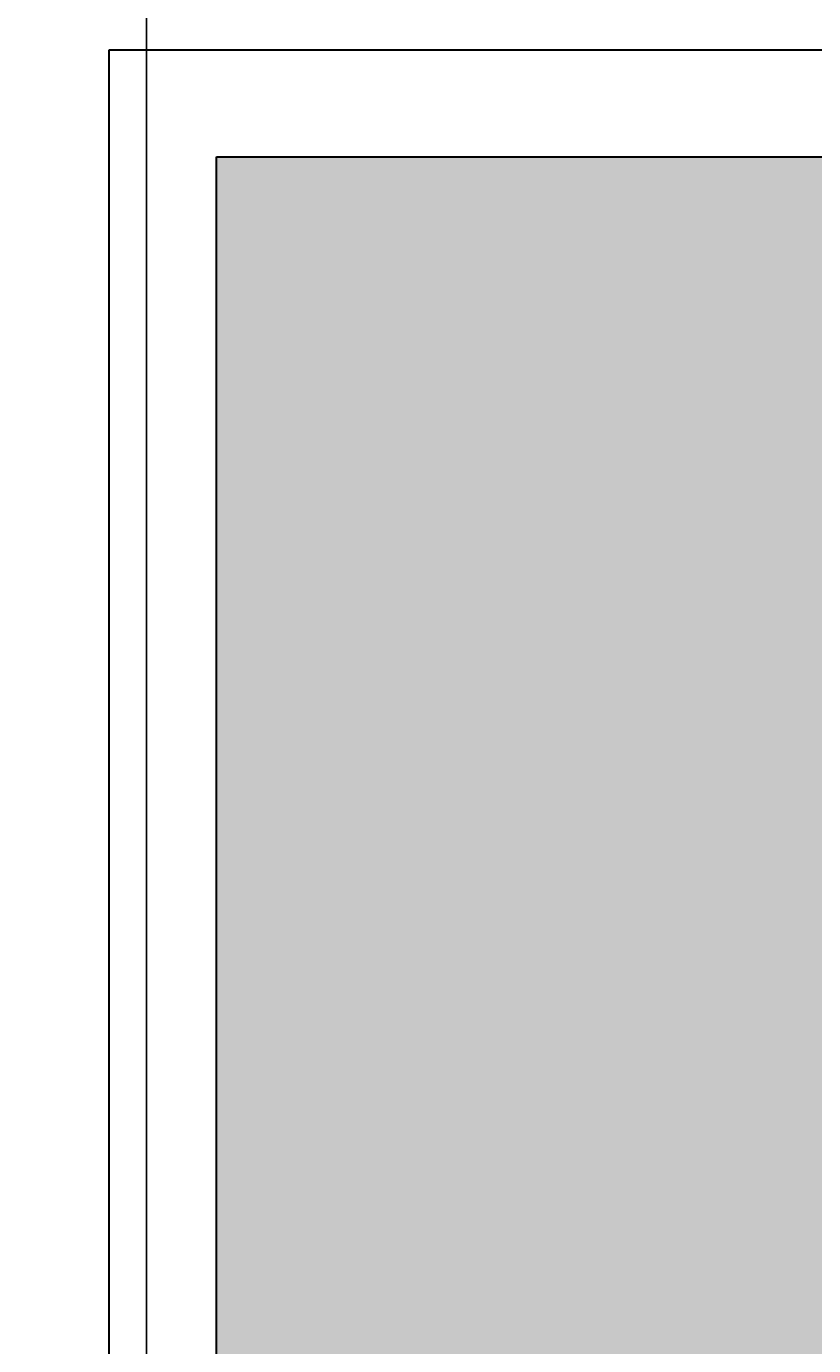
# Model space of a CAD drawing. Units: millimetres. Extents: x -8 to 285, y 5 to 221.
# Tile 19 of 30: x 186 to 208, y 66 to 103. Entities that reach past the tile are written whole.
import ezdxf

# ---------------------------------------------------------------- set-up
doc = ezdxf.new("R2010")
doc.units = ezdxf.units.MM
for name, color, linetype, lineweight in [('A-ANNO-DIMS', 2, 'Continuous', 18), ('E-EQPM-PATT', 252, 'Continuous', 13), ('E-POWR-INVR', 7, 'Continuous', 30)]:
    doc.layers.add(name, color=color, linetype=linetype, lineweight=lineweight)
doc.styles.get("Standard").update_dxf_attribs({"font": 'arial.ttf'})
doc.dimstyles.get("Standard").update_dxf_attribs({"dimtxt": 0.18, "dimasz": 0.18, "dimexe": 0.18, "dimexo": 0.0625, "dimgap": 0.09, "dimtad": 0, "dimtih": 1, "dimtoh": 1, "dimdec": 4, "dimzin": 0, "dimdsep": 46, "dimtxsty": 'Standard', "dimcen": 0.09, "dimadec": 0, "dimazin": 0, "dimtfac": 1, "dimtdec": 4, "dimtofl": 0, "dimtmove": 0, "dimatfit": 3, "dimfxl": 1, "dimtolj": 1, "dimtzin": 0, "dimarcsym": 0})

# ---------------------------------------------------------------- blocks, each defined once
blk = doc.blocks.new('*D13')
at = {"layer": 'A-ANNO-DIMS', "color": 0, "lineweight": -2, "transparency": 16777216}
for p, q in [((145.21, 137.013), (145.21, 5.222)), ((189.039, 137.013), (189.039, 5.222)), ((145.39, 5.402), (166.727, 5.402)), ((188.859, 5.402), (167.522, 5.402))]:
    blk.add_line(p, q, dxfattribs=at)
at = {"layer": 'A-ANNO-DIMS', "color": 0, "transparency": 16777216}
for points in [[(145.39, 5.432), (145.39, 5.372), (145.21, 5.402)], [(188.859, 5.432), (188.859, 5.372), (189.039, 5.402)]]:
    blk.add_solid(points, dxfattribs=at)
at = {"layer": 'Defpoints', "color": 0, "transparency": 16777216}
for p in [(145.21, 137.075), (189.039, 137.075), (189.039, 5.402)]:
    blk.add_point(p, dxfattribs=at)
at = {"layer": 'A-ANNO-DIMS', "color": 0, "transparency": 16777216, "insert": (167.124, 5.402), "char_height": 0.18, "attachment_point": 5}
blk.add_mtext('\\A1;43.83', dxfattribs=at)
blk = doc.blocks.new('*D14')
at = {"layer": 'A-ANNO-DIMS', "color": 0, "lineweight": -2, "transparency": 16777216}
for p, q in [((189.039, 137.013), (189.039, 5.222)), ((230.967, 137.013), (230.967, 5.222)), ((189.219, 5.402), (209.606, 5.402)), ((230.787, 5.402), (210.4, 5.402))]:
    blk.add_line(p, q, dxfattribs=at)
at = {"layer": 'A-ANNO-DIMS', "color": 0, "transparency": 16777216}
for points in [[(189.219, 5.432), (189.219, 5.372), (189.039, 5.402)], [(230.787, 5.432), (230.787, 5.372), (230.967, 5.402)]]:
    blk.add_solid(points, dxfattribs=at)
at = {"layer": 'Defpoints', "color": 0, "transparency": 16777216}
for p in [(189.039, 137.075), (230.967, 137.075), (230.967, 5.402)]:
    blk.add_point(p, dxfattribs=at)
at = {"layer": 'A-ANNO-DIMS', "color": 0, "transparency": 16777216, "insert": (210.003, 5.402), "char_height": 0.18, "attachment_point": 5}
blk.add_mtext('\\A1;41.93', dxfattribs=at)

msp = doc.modelspace()

# ---------------------------------------------------------------- hatches: boundary and pattern name
at = {"layer": 'E-EQPM-PATT'}
h = msp.add_hatch(color=256, dxfattribs=at)
h.set_gradient(color1=(175, 217, 170), color2=(175, 217, 170), tint=1)
h.paths.add_polyline_path([(255.6152, 99.7021), (190.9955, 99.7021), (190.9955, 53.4644), (215.8749, 53.4644), (215.8749, 47.6512), (217.2608, 47.6512), (219.2608, 45.6512), (219.2608, 32.6512), (199.2608, 32.6512), (199.2608, 44.4759), (190.9955, 44.4759), (190.9955, 28.2311), (237.8513, 28.2311), (237.8513, 32.6512), (231.5468, 32.6512, -0.5773503), (229.8147, 35.6512), (231.5468, 38.6512), (231.5468, 58.5666), (255.6152, 58.5666)])
h.paths.add_polyline_path([(208.2775, 92.6953), (238.0827, 92.6953), (238.0827, 67.6708), (208.2775, 67.6708)], flags=16)
h.paths.add_polyline_path([(213.1801, 80.183, -1), (233.1801, 80.183, -1)], flags=0)
h.paths.add_polyline_path([(215.1801, 80.183, -1), (231.1801, 80.183, -1)], flags=0)
h.paths.add_polyline_path([(217.1801, 80.183, -1), (229.1801, 80.183, -1)], flags=0)
h.paths.add_polyline_path([(219.1801, 80.183, -1), (227.1801, 80.183, -1)], flags=0)
h.paths.add_polyline_path([(255.6152, 58.5666), (231.5468, 58.5666), (231.5468, 38.6512), (236.3506, 46.9717, -0.5773503), (239.8147, 46.9717), (244.6186, 38.6512), (244.6186, 49.925), (255.6152, 49.925)], flags=17)
h.paths.add_polyline_path([(215.8749, 53.4644), (190.9955, 53.4644), (190.9955, 48.962), (202.4345, 48.962), (202.4345, 47.6512), (215.8749, 47.6512)], flags=17)
h.paths.add_polyline_path([(255.6152, 49.925), (244.6186, 49.925), (244.6186, 38.6512), (246.3506, 35.6512, -0.5773503), (244.6186, 32.6512), (237.8513, 32.6512), (237.8513, 28.2311), (190.9955, 28.2311), (190.9955, 25.6297), (255.6152, 25.6297)])
h.paths.add_polyline_path([(199.2608, 45.6512), (201.2608, 47.6512), (202.4345, 47.6512), (202.4345, 48.962), (190.9955, 48.962), (190.9955, 44.4759), (199.2608, 44.4759)], flags=17)

# ---------------------------------------------------------------- linework, layer by layer
at = {"layer": 'E-POWR-INVR'}
for points in [[(187.9955, 102.7021), (258.6152, 102.7021), (258.6152, 22.6297), (187.9955, 22.6297)], [(190.9955, 99.7021), (255.6152, 99.7021), (255.6152, 25.6297), (190.9955, 25.6297)]]:
    msp.add_lwpolyline(points, close=True, dxfattribs=at)

# ---------------------------------------------------------------- dimensions: what is measured, and where the dimension line sits
at = {"layer": 'A-ANNO-DIMS'}
for base, p1, p2, picture, middle in [((189.039, 5.402), (145.2095, 137.0752), (189.039, 137.0752), '*D13', (167.1243, 5.402)), ((230.9672, 5.402), (189.039, 137.0752), (230.9672, 137.0752), '*D14', (210.0031, 5.402))]:
    dim = msp.add_linear_dim(base=base, p1=p1, p2=p2, dimstyle='Standard', override={"dimdec": 2, "dimlfac": 1, "dimrnd": 0, "dimzin": 0, "dimdsep": 46, "dimlunit": 2}, dxfattribs=at)
    dim.commit()
    dim.dimension.update_dxf_attribs({"geometry": picture, "text_midpoint": middle})

doc.saveas('drawing.dxf')
